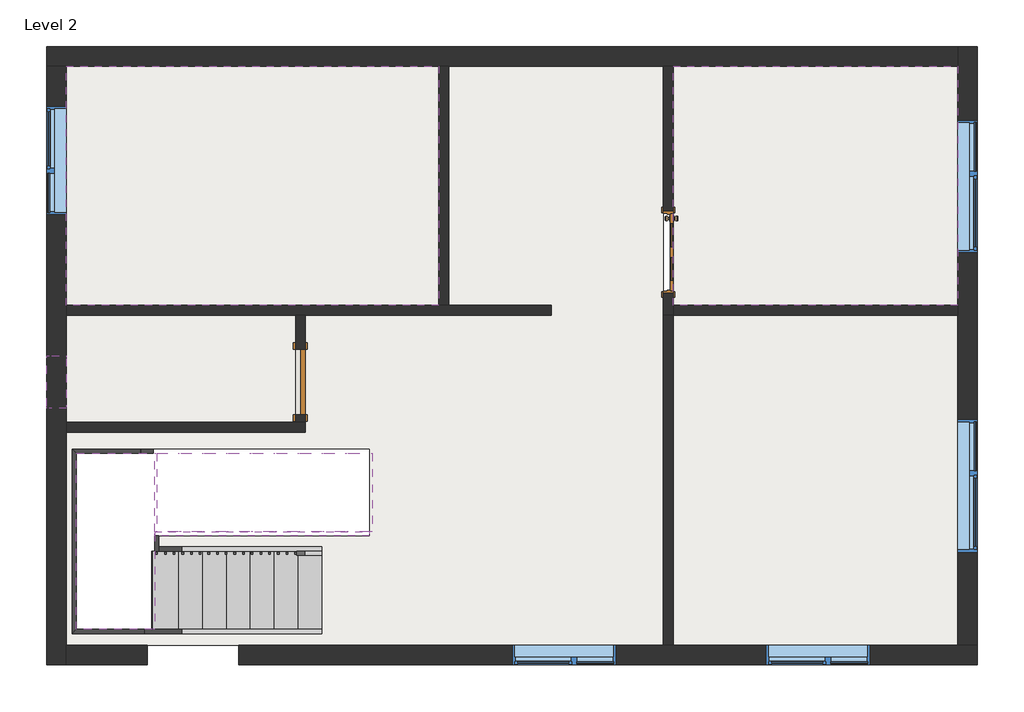
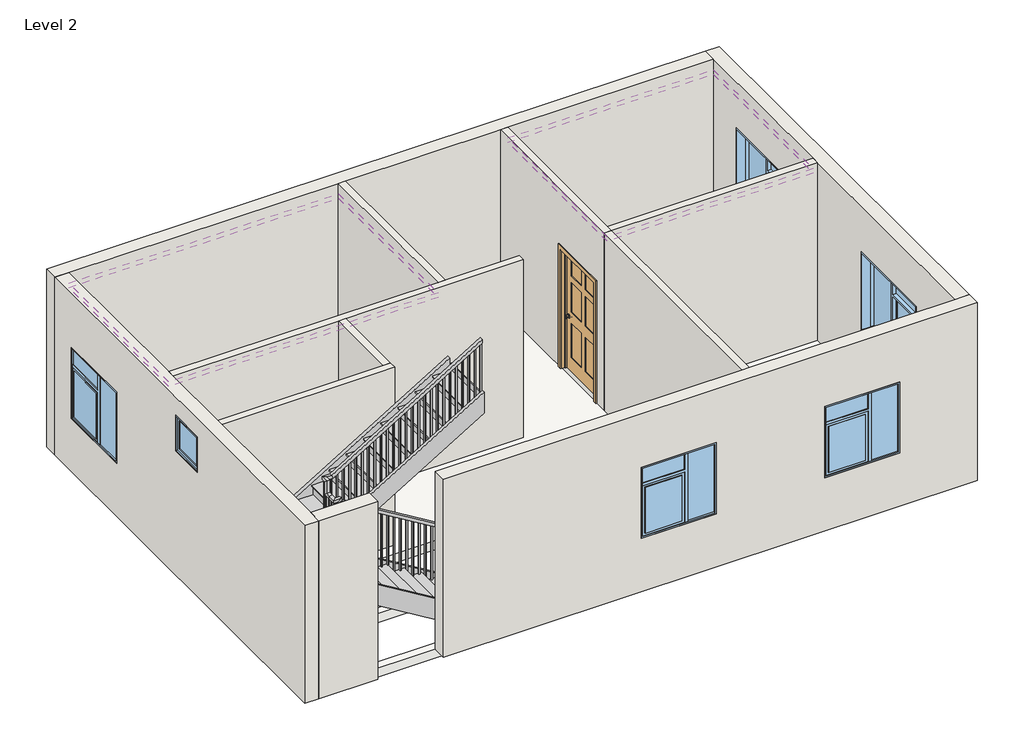
# One storey: 11 walls, 8 members, 6 windows, 4 coverings, 2 doors, 2 slabs, 2 stair flights, 1 railing.
"""IFC4 building model written with IfcOpenShell, lengths in millimetres."""

from ifc_helpers import new_model, si_unit, frame, origin, place, context, project, spatial, polyline, outline, extrude, faceted_brep, transform, mapped, element, save
from components import door_92bad2d9, door_d8f5dbb5, non_monolithic_landing_0199e9fe, stair_flight_13fda11b, stair_flight_c7e5c723, window_80340324, window_ae1cb28a, window_390faff0, window_casement_double_sidelight_windows_4_x_4_2_a48be683

model = new_model("IFC4")

# Units and contexts
model_context = context("Model", 3, world=origin())
ifc_project = project(units=[si_unit("LENGTHUNIT", "METRE", prefix="MILLI")], contexts=[model_context])

# Site, building, storey
site = spatial("IfcSite", under=ifc_project)
building = spatial("IfcBuilding", under=site)
storey = spatial("IfcBuildingStorey", under=building, Name="Level 2", Elevation=3352.8)

# Coverings
placement = place(None, origin())
element("IfcCovering", 1, ObjectType="METAL WHITE CEILING", at=placement, inside=storey, context=model_context, shape_type="SweptSolid", body=[
    extrude(outline(polyline([(-15611.0277023, 6236.3679075), (-11248.5777023, 6236.3679075), (-11248.5777023, 3436.0179075), (-15611.0277023, 3436.0179075), (-15611.0277023, 6236.3679075)])), frame((0.0, 0.0, 6223.0), z_axis=(0.0, 0.0, 1.0), x_axis=(1.0, 0.0, 0.0)), (0.0, 0.0, 1.0), 107.95),
])
element("IfcCovering", 2, ObjectType="METAL WHITE CEILING", at=placement, inside=storey, context=model_context, shape_type="SweptSolid", body=[
    extrude(outline(polyline([(-11248.5777023, 6236.3679075), (-11248.5777023, 3436.0179075), (-15611.0277023, 3436.0179075), (-15611.0277023, 6236.3679075), (-11248.5777023, 6236.3679075)]), holes=[polyline([(-11553.3777023, 5931.5679075), (-15306.2277023, 5931.5679075), (-15306.2277023, 3740.8179075), (-11553.3777023, 3740.8179075), (-11553.3777023, 5931.5679075)])]), frame((0.0, 0.0, 6146.8), z_axis=(0.0, 0.0, 1.0), x_axis=(1.0, 0.0, 0.0)), (0.0, 0.0, 1.0), 107.95),
    extrude(outline(polyline([(-14689.9397973, 5626.7679075), (-14689.9397973, 4045.6179075), (-15001.4277023, 4045.6179075), (-15001.4277023, 5626.7679075), (-14689.9397973, 5626.7679075)])), frame((0.0, 0.0, 6146.8), z_axis=(0.0, 0.0, 1.0), x_axis=(1.0, 0.0, 0.0)), (0.0, 0.0, 1.0), 107.95),
    extrude(outline(polyline([(-14080.3397973, 5626.7679075), (-14080.3397973, 4045.6179075), (-14391.8277023, 4045.6179075), (-14391.8277023, 5626.7679075), (-14080.3397973, 5626.7679075)])), frame((0.0, 0.0, 6146.8), z_axis=(0.0, 0.0, 1.0), x_axis=(1.0, 0.0, 0.0)), (0.0, 0.0, 1.0), 107.95),
    extrude(outline(polyline([(-13470.7397973, 5626.7679075), (-13470.7397973, 4045.6179075), (-13782.2277023, 4045.6179075), (-13782.2277023, 5626.7679075), (-13470.7397973, 5626.7679075)])), frame((0.0, 0.0, 6146.8), z_axis=(0.0, 0.0, 1.0), x_axis=(1.0, 0.0, 0.0)), (0.0, 0.0, 1.0), 107.95),
    extrude(outline(polyline([(-12861.1397973, 5626.7679075), (-12861.1397973, 4045.6179075), (-13172.6277023, 4045.6179075), (-13172.6277023, 5626.7679075), (-12861.1397973, 5626.7679075)])), frame((0.0, 0.0, 6146.8), z_axis=(0.0, 0.0, 1.0), x_axis=(1.0, 0.0, 0.0)), (0.0, 0.0, 1.0), 107.95),
    extrude(outline(polyline([(-12251.5397973, 5626.7679075), (-12251.5397973, 4045.6179075), (-12563.0277023, 4045.6179075), (-12563.0277023, 5626.7679075), (-12251.5397973, 5626.7679075)])), frame((0.0, 0.0, 6146.8), z_axis=(0.0, 0.0, 1.0), x_axis=(1.0, 0.0, 0.0)), (0.0, 0.0, 1.0), 107.95),
    extrude(outline(polyline([(-11641.9397973, 5626.7679075), (-11641.9397973, 4045.6179075), (-11953.4277023, 4045.6179075), (-11953.4277023, 5626.7679075), (-11641.9397973, 5626.7679075)])), frame((0.0, 0.0, 6146.8), z_axis=(0.0, 0.0, 1.0), x_axis=(1.0, 0.0, 0.0)), (0.0, 0.0, 1.0), 107.95),
])
element("IfcCovering", 3, ObjectType="METAL WHITE CEILING", at=placement, inside=storey, context=model_context, shape_type="SweptSolid", body=[
    extrude(outline(polyline([(-8505.3777023, 3436.0179075), (-8505.3777023, 6236.3679075), (-5171.6277023, 6236.3679075), (-5171.6277023, 3436.0179075), (-8505.3777023, 3436.0179075)])), frame((0.0, 0.0, 6223.0), z_axis=(0.0, 0.0, 1.0), x_axis=(1.0, 0.0, 0.0)), (0.0, 0.0, 1.0), 107.95),
])
element("IfcCovering", 4, ObjectType="METAL WHITE CEILING", at=placement, inside=storey, context=model_context, shape_type="SweptSolid", body=[
    extrude(outline(polyline([(-5171.6277023, 6236.3679075), (-5171.6277023, 3436.0179075), (-8505.3777023, 3436.0179075), (-8505.3777023, 6236.3679075), (-5171.6277023, 6236.3679075)]), holes=[polyline([(-5476.4277023, 5931.5679075), (-8200.5777023, 5931.5679075), (-8200.5777023, 3740.8179075), (-5476.4277023, 3740.8179075), (-5476.4277023, 5931.5679075)])]), frame((0.0, 0.0, 6146.8), z_axis=(0.0, 0.0, 1.0), x_axis=(1.0, 0.0, 0.0)), (0.0, 0.0, 1.0), 107.95),
    extrude(outline(polyline([(-7575.2115209, 5626.7679075), (-7575.2115209, 4045.6179075), (-7880.0115209, 4045.6179075), (-7880.0115209, 5626.7679075), (-7575.2115209, 5626.7679075)])), frame((0.0, 0.0, 6146.8), z_axis=(0.0, 0.0, 1.0), x_axis=(1.0, 0.0, 0.0)), (0.0, 0.0, 1.0), 107.95),
    extrude(outline(polyline([(-6965.6115209, 5626.7679075), (-6965.6115209, 4045.6179075), (-7270.4115209, 4045.6179075), (-7270.4115209, 5626.7679075), (-6965.6115209, 5626.7679075)])), frame((0.0, 0.0, 6146.8), z_axis=(0.0, 0.0, 1.0), x_axis=(1.0, 0.0, 0.0)), (0.0, 0.0, 1.0), 107.95),
    extrude(outline(polyline([(-6356.0115209, 5626.7679075), (-6356.0115209, 4045.6179075), (-6660.8115209, 4045.6179075), (-6660.8115209, 5626.7679075), (-6356.0115209, 5626.7679075)])), frame((0.0, 0.0, 6146.8), z_axis=(0.0, 0.0, 1.0), x_axis=(1.0, 0.0, 0.0)), (0.0, 0.0, 1.0), 107.95),
    extrude(outline(polyline([(-5746.4115209, 5626.7679075), (-5746.4115209, 4045.6179075), (-6051.2115209, 4045.6179075), (-6051.2115209, 5626.7679075), (-5746.4115209, 5626.7679075)])), frame((0.0, 0.0, 6146.8), z_axis=(0.0, 0.0, 1.0), x_axis=(1.0, 0.0, 0.0)), (0.0, 0.0, 1.0), 107.95),
])

# Doors
door_shape = door_92bad2d9(model_context)
element("IfcDoor", 5, ObjectType="Door-Interior-Single-6_Panel-Wood : 36\" x 80\"", at=placement, inside=storey, context=model_context, shape_type="MappedRepresentation", body=[
    mapped(door_shape, transform((-8559.3527023, 4058.3179075, 3352.8), x_axis=(0.0, -1.0, 0.0), y_axis=(1.0, 0.0, 0.0), z_axis=(0.0, 0.0, 1.0))),
])
door_2_shape = door_d8f5dbb5(model_context)
element("IfcDoor", 6, ObjectType="Single-Flush : 30\" x 80\"", at=placement, inside=storey, context=model_context, shape_type="MappedRepresentation", body=[
    mapped(door_2_shape, transform((-12867.8277023, 2538.826922, 3386.2495969), x_axis=(0.0, -1.0, 0.0), y_axis=(1.0, 0.0, 0.0), z_axis=(0.0, 0.0, 1.0))),
])

# Members
element("IfcMember", 7, ObjectType="Stringer - 2\" Width", at=placement, inside=storey, context=model_context, shape_type="SweptSolid", body=[
    extrude(outline(polyline([(3352.8, -12620.1777023), (3564.914512, -12620.1777023), (4783.6666667, -14631.1187576), (4478.8666667, -14716.2732141), (3352.8, -12858.2632141), (3352.8, -12620.1777023)])), frame((0.0, -405.7320925, 0.0), z_axis=(0.0, 1.0, 0.0), x_axis=(0.0, 0.0, 1.0)), (0.0, 0.0, 1.0), 50.8),
])
element("IfcMember", 8, ObjectType="Stringer - 2\" Width", at=placement, inside=storey, context=model_context, shape_type="SweptSolid", body=[
    extrude(outline(polyline([(3352.8, -12620.1777023), (3564.914512, -12620.1777023), (4719.4599665, -14525.1777023), (4363.051205, -14525.1777023), (3352.8, -12858.2632141), (3352.8, -12620.1777023)])), frame((0.0, 559.4679075, 0.0), z_axis=(0.0, 1.0, 0.0), x_axis=(0.0, 0.0, 1.0)), (0.0, 0.0, 1.0), 50.8),
])
element("IfcMember", 9, ObjectType="Stringer - 2\" Width", at=placement, inside=storey, context=model_context, shape_type="SweptSolid", body=[
    extrude(outline(polyline([(4783.6666667, -14800.2366471), (4478.8666667, -14715.0821905), (6087.1724171, -12061.3777023), (6443.5811786, -12061.3777023), (4783.6666667, -14800.2366471)])), frame((0.0, 1702.4679075, 0.0), z_axis=(0.0, 1.0, 0.0), x_axis=(0.0, 0.0, 1.0)), (0.0, 0.0, 1.0), 50.8),
])
element("IfcMember", 10, ObjectType="Stringer - 2\" Width", at=placement, inside=storey, context=model_context, shape_type="SweptSolid", body=[
    extrude(outline(polyline([(4919.5811786, -14575.9777023), (4563.1724171, -14575.9777023), (6087.1724171, -12061.3777023), (6443.5811786, -12061.3777023), (4919.5811786, -14575.9777023)])), frame((0.0, 737.2679075, 0.0), z_axis=(0.0, 1.0, 0.0), x_axis=(0.0, 0.0, 1.0)), (0.0, 0.0, 1.0), 50.8),
])
element("IfcMember", 11, ObjectType="Stringer - 2\" Width", at=placement, inside=storey, context=model_context, shape_type="Brep", body=[
    faceted_brep([(-14800.2366471, 1702.4679075, 4783.6666667), (-14800.2366471, 1753.2679075, 4783.6666667), (-15541.1777023, 1753.2679075, 4783.6666667), (-15490.3777023, 1702.4679075, 4783.6666667), (-14715.0821905, 1702.4679075, 4478.8666667), (-15490.3777023, 1702.4679075, 4478.8666667), (-14715.0821905, 1753.2679075, 4478.8666667), (-15541.1777023, 1753.2679075, 4478.8666667)], [[[0, 1, 2, 3]], [[4, 0, 3, 5]], [[6, 4, 5, 7]], [[1, 6, 7, 2]], [[1, 0, 4, 6]], [[2, 7, 5, 3]]]),
])
element("IfcMember", 12, ObjectType="Stringer - 2\" Width", at=placement, inside=storey, context=model_context, shape_type="SweptSolid", body=[
    extrude(outline(polyline([(-15541.1777023, 1753.2679075), (-15490.3777023, 1702.4679075), (-15490.3777023, -354.9320925), (-15541.1777023, -405.7320925), (-15541.1777023, 1753.2679075)])), frame((0.0, 0.0, 4478.8666667), z_axis=(0.0, 0.0, 1.0), x_axis=(1.0, 0.0, 0.0)), (0.0, 0.0, 1.0), 304.8),
])
element("IfcMember", 13, ObjectType="Stringer - 2\" Width", at=placement, inside=storey, context=model_context, shape_type="Brep", body=[
    faceted_brep([(-15490.3777023, -354.9320925, 4783.6666667), (-15541.1777023, -405.7320925, 4783.6666667), (-14631.1187576, -405.7320925, 4783.6666667), (-14631.1187576, -354.9320925, 4783.6666667), (-15490.3777023, -354.9320925, 4478.8666667), (-14716.2732141, -354.9320925, 4478.8666667), (-15541.1777023, -405.7320925, 4478.8666667), (-14716.2732141, -405.7320925, 4478.8666667)], [[[0, 1, 2, 3]], [[4, 0, 3, 5]], [[6, 4, 5, 7]], [[1, 6, 7, 2]], [[1, 0, 4, 6]], [[2, 7, 5, 3]]]),
])
element("IfcMember", 14, ObjectType="Stringer - 2\" Width", at=placement, inside=storey, context=model_context, shape_type="SweptSolid", body=[
    extrude(outline(polyline([(-14525.1777023, 559.4679075), (-14575.9777023, 559.4679075), (-14575.9777023, 737.2679075), (-14525.1777023, 737.2679075), (-14525.1777023, 559.4679075)])), frame((0.0, 0.0, 4478.8666667), z_axis=(0.0, 0.0, 1.0), x_axis=(1.0, 0.0, 0.0)), (0.0, 0.0, 1.0), 304.8),
])

# Railing
element("IfcRailing", 15, ObjectType="Handrail - Rectangular", at=placement, inside=storey, context=model_context, shape_type="SolidModel", body=[
    faceted_brep([(-12620.1777023, 508.6679075, 4436.5333333), (-12620.1777023, 508.6679075, 4377.1318731), (-12620.1777023, 559.4679075, 4377.1318731), (-12620.1777023, 559.4679075, 4436.5333333), (-14499.7777023, 508.6679075, 5575.6848485), (-14550.5777023, 508.6679075, 5547.071267), (-14550.5777023, 559.4679075, 5547.071267), (-14499.7777023, 559.4679075, 5575.6848485), (-14499.7777023, 508.6679075, 5621.8666667), (-14550.5777023, 508.6679075, 5571.0666667), (-14550.5777023, 559.4679075, 5571.0666667), (-14499.7777023, 559.4679075, 5621.8666667), (-14626.7777023, 508.6679075, 5621.8666667), (-14626.7777023, 508.6679075, 5571.0666667), (-14575.9777023, 559.4679075, 5571.0666667), (-14575.9777023, 559.4679075, 5621.8666667), (-14626.7777023, 635.6679075, 5621.8666667), (-14626.7777023, 635.6679075, 5571.0666667), (-14575.9777023, 635.6679075, 5571.0666667), (-14575.9777023, 635.6679075, 5621.8666667), (-14626.7777023, 711.8679075, 5621.8666667), (-14626.7777023, 762.6679075, 5571.0666667), (-14575.9777023, 762.6679075, 5571.0666667), (-14575.9777023, 711.8679075, 5621.8666667), (-14626.7777023, 711.8679075, 5837.3818182), (-14626.7777023, 762.6679075, 5786.5818182), (-14575.9777023, 762.6679075, 5786.5818182), (-14575.9777023, 711.8679075, 5837.3818182), (-14626.7777023, 838.8679075, 5837.3818182), (-14626.7777023, 838.8679075, 5786.5818182), (-14575.9777023, 788.0679075, 5786.5818182), (-14575.9777023, 788.0679075, 5837.3818182), (-14499.7777023, 838.8679075, 5837.3818182), (-14485.5852929, 838.8679075, 5786.5818182), (-14485.5852929, 788.0679075, 5786.5818182), (-14499.7777023, 788.0679075, 5837.3818182), (-12061.3777023, 838.8679075, 7315.2), (-12061.3777023, 788.0679075, 7315.2), (-12061.3777023, 788.0679075, 7255.7985397), (-12061.3777023, 838.8679075, 7255.7985397)], [[[0, 1, 2, 3]], [[1, 0, 4, 5]], [[2, 1, 5, 6]], [[3, 2, 6, 7]], [[0, 3, 7, 4]], [[5, 4, 8, 9]], [[6, 5, 9, 10]], [[7, 6, 10, 11]], [[4, 7, 11, 8]], [[9, 8, 12, 13]], [[10, 9, 13, 14]], [[11, 10, 14, 15]], [[8, 11, 15, 12]], [[13, 12, 16, 17]], [[14, 13, 17, 18]], [[15, 14, 18, 19]], [[12, 15, 19, 16]], [[17, 16, 20, 21]], [[18, 17, 21, 22]], [[19, 18, 22, 23]], [[16, 19, 23, 20]], [[21, 20, 24, 25]], [[22, 21, 25, 26]], [[23, 22, 26, 27]], [[20, 23, 27, 24]], [[25, 24, 28, 29]], [[26, 25, 29, 30]], [[27, 26, 30, 31]], [[24, 27, 31, 28]], [[29, 28, 32, 33]], [[30, 29, 33, 34]], [[31, 30, 34, 35]], [[28, 31, 35, 32]], [[36, 37, 38, 39]], [[33, 32, 36, 39]], [[34, 33, 39, 38]], [[35, 34, 38, 37]], [[32, 35, 37, 36]]]),
    extrude(outline(polyline([(7199.9955094, -12153.4527023), (7188.4500549, -12172.5027023), (6231.4666667, -12172.5027023), (6231.4666667, -12153.4527023), (7199.9955094, -12153.4527023)])), frame((0.0, 803.9429075, 0.0), z_axis=(0.0, 1.0, 0.0), x_axis=(0.0, 0.0, 1.0)), (0.0, 0.0, 1.0), 19.05),
    extrude(outline(polyline([(7138.4197519, -12255.0527023), (7126.8742973, -12274.1027023), (6231.4666667, -12274.1027023), (6231.4666667, -12255.0527023), (7138.4197519, -12255.0527023)])), frame((0.0, 803.9429075, 0.0), z_axis=(0.0, 1.0, 0.0), x_axis=(0.0, 0.0, 1.0)), (0.0, 0.0, 1.0), 19.05),
    extrude(outline(polyline([(7076.8439943, -12356.6527023), (7065.2985397, -12375.7027023), (6062.1333333, -12375.7027023), (6062.1333333, -12356.6527023), (7076.8439943, -12356.6527023)])), frame((0.0, 803.9429075, 0.0), z_axis=(0.0, 1.0, 0.0), x_axis=(0.0, 0.0, 1.0)), (0.0, 0.0, 1.0), 19.05),
    extrude(outline(polyline([(7015.2682367, -12458.2527023), (7003.7227822, -12477.3027023), (6062.1333333, -12477.3027023), (6062.1333333, -12458.2527023), (7015.2682367, -12458.2527023)])), frame((0.0, 803.9429075, 0.0), z_axis=(0.0, 1.0, 0.0), x_axis=(0.0, 0.0, 1.0)), (0.0, 0.0, 1.0), 19.05),
    extrude(outline(polyline([(6953.6924791, -12559.8527023), (6942.1470246, -12578.9027023), (6062.1333333, -12578.9027023), (6062.1333333, -12559.8527023), (6953.6924791, -12559.8527023)])), frame((0.0, 803.9429075, 0.0), z_axis=(0.0, 1.0, 0.0), x_axis=(0.0, 0.0, 1.0)), (0.0, 0.0, 1.0), 19.05),
    extrude(outline(polyline([(6892.1167216, -12661.4527023), (6880.571267, -12680.5027023), (5892.8, -12680.5027023), (5892.8, -12661.4527023), (6892.1167216, -12661.4527023)])), frame((0.0, 803.9429075, 0.0), z_axis=(0.0, 1.0, 0.0), x_axis=(0.0, 0.0, 1.0)), (0.0, 0.0, 1.0), 19.05),
    extrude(outline(polyline([(6830.540964, -12763.0527023), (6818.9955094, -12782.1027023), (5892.8, -12782.1027023), (5892.8, -12763.0527023), (6830.540964, -12763.0527023)])), frame((0.0, 803.9429075, 0.0), z_axis=(0.0, 1.0, 0.0), x_axis=(0.0, 0.0, 1.0)), (0.0, 0.0, 1.0), 19.05),
    extrude(outline(polyline([(6768.9652064, -12864.6527023), (6757.4197519, -12883.7027023), (5892.8, -12883.7027023), (5892.8, -12864.6527023), (6768.9652064, -12864.6527023)])), frame((0.0, 803.9429075, 0.0), z_axis=(0.0, 1.0, 0.0), x_axis=(0.0, 0.0, 1.0)), (0.0, 0.0, 1.0), 19.05),
    extrude(outline(polyline([(6707.3894488, -12966.2527023), (6695.8439943, -12985.3027023), (5723.4666667, -12985.3027023), (5723.4666667, -12966.2527023), (6707.3894488, -12966.2527023)])), frame((0.0, 803.9429075, 0.0), z_axis=(0.0, 1.0, 0.0), x_axis=(0.0, 0.0, 1.0)), (0.0, 0.0, 1.0), 19.05),
    extrude(outline(polyline([(6645.8136913, -13067.8527023), (6634.2682367, -13086.9027023), (5723.4666667, -13086.9027023), (5723.4666667, -13067.8527023), (6645.8136913, -13067.8527023)])), frame((0.0, 803.9429075, 0.0), z_axis=(0.0, 1.0, 0.0), x_axis=(0.0, 0.0, 1.0)), (0.0, 0.0, 1.0), 19.05),
    extrude(outline(polyline([(6584.2379337, -13169.4527023), (6572.6924791, -13188.5027023), (5723.4666667, -13188.5027023), (5723.4666667, -13169.4527023), (6584.2379337, -13169.4527023)])), frame((0.0, 803.9429075, 0.0), z_axis=(0.0, 1.0, 0.0), x_axis=(0.0, 0.0, 1.0)), (0.0, 0.0, 1.0), 19.05),
    extrude(outline(polyline([(6522.6621761, -13271.0527023), (6511.1167216, -13290.1027023), (5554.1333333, -13290.1027023), (5554.1333333, -13271.0527023), (6522.6621761, -13271.0527023)])), frame((0.0, 803.9429075, 0.0), z_axis=(0.0, 1.0, 0.0), x_axis=(0.0, 0.0, 1.0)), (0.0, 0.0, 1.0), 19.05),
    extrude(outline(polyline([(6461.0864185, -13372.6527023), (6449.540964, -13391.7027023), (5554.1333333, -13391.7027023), (5554.1333333, -13372.6527023), (6461.0864185, -13372.6527023)])), frame((0.0, 803.9429075, 0.0), z_axis=(0.0, 1.0, 0.0), x_axis=(0.0, 0.0, 1.0)), (0.0, 0.0, 1.0), 19.05),
    extrude(outline(polyline([(6399.510661, -13474.2527023), (6387.9652064, -13493.3027023), (5384.8, -13493.3027023), (5384.8, -13474.2527023), (6399.510661, -13474.2527023)])), frame((0.0, 803.9429075, 0.0), z_axis=(0.0, 1.0, 0.0), x_axis=(0.0, 0.0, 1.0)), (0.0, 0.0, 1.0), 19.05),
    extrude(outline(polyline([(6337.9349034, -13575.8527023), (6326.3894488, -13594.9027023), (5384.8, -13594.9027023), (5384.8, -13575.8527023), (6337.9349034, -13575.8527023)])), frame((0.0, 803.9429075, 0.0), z_axis=(0.0, 1.0, 0.0), x_axis=(0.0, 0.0, 1.0)), (0.0, 0.0, 1.0), 19.05),
    extrude(outline(polyline([(6276.3591458, -13677.4527023), (6264.8136913, -13696.5027023), (5384.8, -13696.5027023), (5384.8, -13677.4527023), (6276.3591458, -13677.4527023)])), frame((0.0, 803.9429075, 0.0), z_axis=(0.0, 1.0, 0.0), x_axis=(0.0, 0.0, 1.0)), (0.0, 0.0, 1.0), 19.05),
    extrude(outline(polyline([(6214.7833882, -13779.0527023), (6203.2379337, -13798.1027023), (5215.4666667, -13798.1027023), (5215.4666667, -13779.0527023), (6214.7833882, -13779.0527023)])), frame((0.0, 803.9429075, 0.0), z_axis=(0.0, 1.0, 0.0), x_axis=(0.0, 0.0, 1.0)), (0.0, 0.0, 1.0), 19.05),
    extrude(outline(polyline([(6153.2076307, -13880.6527023), (6141.6621761, -13899.7027023), (5215.4666667, -13899.7027023), (5215.4666667, -13880.6527023), (6153.2076307, -13880.6527023)])), frame((0.0, 803.9429075, 0.0), z_axis=(0.0, 1.0, 0.0), x_axis=(0.0, 0.0, 1.0)), (0.0, 0.0, 1.0), 19.05),
    extrude(outline(polyline([(6091.6318731, -13982.2527023), (6080.0864185, -14001.3027023), (5215.4666667, -14001.3027023), (5215.4666667, -13982.2527023), (6091.6318731, -13982.2527023)])), frame((0.0, 803.9429075, 0.0), z_axis=(0.0, 1.0, 0.0), x_axis=(0.0, 0.0, 1.0)), (0.0, 0.0, 1.0), 19.05),
    extrude(outline(polyline([(6030.0561155, -14083.8527023), (6018.510661, -14102.9027023), (5046.1333333, -14102.9027023), (5046.1333333, -14083.8527023), (6030.0561155, -14083.8527023)])), frame((0.0, 803.9429075, 0.0), z_axis=(0.0, 1.0, 0.0), x_axis=(0.0, 0.0, 1.0)), (0.0, 0.0, 1.0), 19.05),
    extrude(outline(polyline([(5968.4803579, -14185.4527023), (5956.9349034, -14204.5027023), (5046.1333333, -14204.5027023), (5046.1333333, -14185.4527023), (5968.4803579, -14185.4527023)])), frame((0.0, 803.9429075, 0.0), z_axis=(0.0, 1.0, 0.0), x_axis=(0.0, 0.0, 1.0)), (0.0, 0.0, 1.0), 19.05),
    extrude(outline(polyline([(5906.9046004, -14287.0527023), (5895.3591458, -14306.1027023), (5046.1333333, -14306.1027023), (5046.1333333, -14287.0527023), (5906.9046004, -14287.0527023)])), frame((0.0, 803.9429075, 0.0), z_axis=(0.0, 1.0, 0.0), x_axis=(0.0, 0.0, 1.0)), (0.0, 0.0, 1.0), 19.05),
    extrude(outline(polyline([(5845.3288428, -14388.6527023), (5833.7833882, -14407.7027023), (4876.8, -14407.7027023), (4876.8, -14388.6527023), (5845.3288428, -14388.6527023)])), frame((0.0, 803.9429075, 0.0), z_axis=(0.0, 1.0, 0.0), x_axis=(0.0, 0.0, 1.0)), (0.0, 0.0, 1.0), 19.05),
    extrude(outline(polyline([(5783.7530852, -14490.2527023), (5772.2076307, -14509.3027023), (4876.8, -14509.3027023), (4876.8, -14490.2527023), (5783.7530852, -14490.2527023)])), frame((0.0, 803.9429075, 0.0), z_axis=(0.0, 1.0, 0.0), x_axis=(0.0, 0.0, 1.0)), (0.0, 0.0, 1.0), 19.05),
    extrude(outline(polyline([(-14591.8527023, 727.7429075), (-14610.9027023, 727.7429075), (-14610.9027023, 746.7929075), (-14591.8527023, 746.7929075), (-14591.8527023, 727.7429075)])), frame((0.0, 0.0, 4707.4666667), z_axis=(0.0, 0.0, 1.0), x_axis=(1.0, 0.0, 0.0)), (0.0, 0.0, 1.0), 1079.1151515),
    extrude(outline(polyline([(-14591.8527023, 626.1429075), (-14610.9027023, 626.1429075), (-14610.9027023, 645.1929075), (-14591.8527023, 645.1929075), (-14591.8527023, 626.1429075)])), frame((0.0, 0.0, 4707.4666667), z_axis=(0.0, 0.0, 1.0), x_axis=(1.0, 0.0, 0.0)), (0.0, 0.0, 1.0), 863.6),
    extrude(outline(polyline([(-14541.0527023, 543.5929075), (-14541.0527023, 524.5429075), (-14560.1027023, 524.5429075), (-14560.1027023, 543.5929075), (-14541.0527023, 543.5929075)])), frame((0.0, 0.0, 4538.1333333), z_axis=(0.0, 0.0, 1.0), x_axis=(1.0, 0.0, 0.0)), (0.0, 0.0, 1.0), 1032.9333333),
    extrude(outline(polyline([(5479.7227822, -14439.4527023), (5491.2682367, -14458.5027023), (4538.1333333, -14458.5027023), (4538.1333333, -14439.4527023), (5479.7227822, -14439.4527023)])), frame((0.0, 524.5429075, 0.0), z_axis=(0.0, 1.0, 0.0), x_axis=(0.0, 0.0, 1.0)), (0.0, 0.0, 1.0), 19.05),
    extrude(outline(polyline([(5418.1470246, -14337.8527023), (5429.6924791, -14356.9027023), (4538.1333333, -14356.9027023), (4538.1333333, -14337.8527023), (5418.1470246, -14337.8527023)])), frame((0.0, 524.5429075, 0.0), z_axis=(0.0, 1.0, 0.0), x_axis=(0.0, 0.0, 1.0)), (0.0, 0.0, 1.0), 19.05),
    extrude(outline(polyline([(5356.571267, -14236.2527023), (5368.1167216, -14255.3027023), (4368.8, -14255.3027023), (4368.8, -14236.2527023), (5356.571267, -14236.2527023)])), frame((0.0, 524.5429075, 0.0), z_axis=(0.0, 1.0, 0.0), x_axis=(0.0, 0.0, 1.0)), (0.0, 0.0, 1.0), 19.05),
    extrude(outline(polyline([(5294.9955094, -14134.6527023), (5306.540964, -14153.7027023), (4368.8, -14153.7027023), (4368.8, -14134.6527023), (5294.9955094, -14134.6527023)])), frame((0.0, 524.5429075, 0.0), z_axis=(0.0, 1.0, 0.0), x_axis=(0.0, 0.0, 1.0)), (0.0, 0.0, 1.0), 19.05),
    extrude(outline(polyline([(5233.4197519, -14033.0527023), (5244.9652064, -14052.1027023), (4368.8, -14052.1027023), (4368.8, -14033.0527023), (5233.4197519, -14033.0527023)])), frame((0.0, 524.5429075, 0.0), z_axis=(0.0, 1.0, 0.0), x_axis=(0.0, 0.0, 1.0)), (0.0, 0.0, 1.0), 19.05),
    extrude(outline(polyline([(5171.8439943, -13931.4527023), (5183.3894488, -13950.5027023), (4199.4666667, -13950.5027023), (4199.4666667, -13931.4527023), (5171.8439943, -13931.4527023)])), frame((0.0, 524.5429075, 0.0), z_axis=(0.0, 1.0, 0.0), x_axis=(0.0, 0.0, 1.0)), (0.0, 0.0, 1.0), 19.05),
    extrude(outline(polyline([(5110.2682367, -13829.8527023), (5121.8136913, -13848.9027023), (4199.4666667, -13848.9027023), (4199.4666667, -13829.8527023), (5110.2682367, -13829.8527023)])), frame((0.0, 524.5429075, 0.0), z_axis=(0.0, 1.0, 0.0), x_axis=(0.0, 0.0, 1.0)), (0.0, 0.0, 1.0), 19.05),
    extrude(outline(polyline([(5048.6924791, -13728.2527023), (5060.2379337, -13747.3027023), (4199.4666667, -13747.3027023), (4199.4666667, -13728.2527023), (5048.6924791, -13728.2527023)])), frame((0.0, 524.5429075, 0.0), z_axis=(0.0, 1.0, 0.0), x_axis=(0.0, 0.0, 1.0)), (0.0, 0.0, 1.0), 19.05),
    extrude(outline(polyline([(4987.1167216, -13626.6527023), (4998.6621761, -13645.7027023), (4030.1333333, -13645.7027023), (4030.1333333, -13626.6527023), (4987.1167216, -13626.6527023)])), frame((0.0, 524.5429075, 0.0), z_axis=(0.0, 1.0, 0.0), x_axis=(0.0, 0.0, 1.0)), (0.0, 0.0, 1.0), 19.05),
    extrude(outline(polyline([(4925.540964, -13525.0527023), (4937.0864185, -13544.1027023), (4030.1333333, -13544.1027023), (4030.1333333, -13525.0527023), (4925.540964, -13525.0527023)])), frame((0.0, 524.5429075, 0.0), z_axis=(0.0, 1.0, 0.0), x_axis=(0.0, 0.0, 1.0)), (0.0, 0.0, 1.0), 19.05),
    extrude(outline(polyline([(4863.9652064, -13423.4527023), (4875.510661, -13442.5027023), (3860.8, -13442.5027023), (3860.8, -13423.4527023), (4863.9652064, -13423.4527023)])), frame((0.0, 524.5429075, 0.0), z_axis=(0.0, 1.0, 0.0), x_axis=(0.0, 0.0, 1.0)), (0.0, 0.0, 1.0), 19.05),
    extrude(outline(polyline([(4802.3894488, -13321.8527023), (4813.9349034, -13340.9027023), (3860.8, -13340.9027023), (3860.8, -13321.8527023), (4802.3894488, -13321.8527023)])), frame((0.0, 524.5429075, 0.0), z_axis=(0.0, 1.0, 0.0), x_axis=(0.0, 0.0, 1.0)), (0.0, 0.0, 1.0), 19.05),
    extrude(outline(polyline([(4740.8136913, -13220.2527023), (4752.3591458, -13239.3027023), (3860.8, -13239.3027023), (3860.8, -13220.2527023), (4740.8136913, -13220.2527023)])), frame((0.0, 524.5429075, 0.0), z_axis=(0.0, 1.0, 0.0), x_axis=(0.0, 0.0, 1.0)), (0.0, 0.0, 1.0), 19.05),
    extrude(outline(polyline([(4679.2379337, -13118.6527023), (4690.7833882, -13137.7027023), (3691.4666667, -13137.7027023), (3691.4666667, -13118.6527023), (4679.2379337, -13118.6527023)])), frame((0.0, 524.5429075, 0.0), z_axis=(0.0, 1.0, 0.0), x_axis=(0.0, 0.0, 1.0)), (0.0, 0.0, 1.0), 19.05),
    extrude(outline(polyline([(4617.6621761, -13017.0527023), (4629.2076307, -13036.1027023), (3691.4666667, -13036.1027023), (3691.4666667, -13017.0527023), (4617.6621761, -13017.0527023)])), frame((0.0, 524.5429075, 0.0), z_axis=(0.0, 1.0, 0.0), x_axis=(0.0, 0.0, 1.0)), (0.0, 0.0, 1.0), 19.05),
    extrude(outline(polyline([(4556.0864185, -12915.4527023), (4567.6318731, -12934.5027023), (3691.4666667, -12934.5027023), (3691.4666667, -12915.4527023), (4556.0864185, -12915.4527023)])), frame((0.0, 524.5429075, 0.0), z_axis=(0.0, 1.0, 0.0), x_axis=(0.0, 0.0, 1.0)), (0.0, 0.0, 1.0), 19.05),
    extrude(outline(polyline([(4494.510661, -12813.8527023), (4506.0561155, -12832.9027023), (3522.1333333, -12832.9027023), (3522.1333333, -12813.8527023), (4494.510661, -12813.8527023)])), frame((0.0, 524.5429075, 0.0), z_axis=(0.0, 1.0, 0.0), x_axis=(0.0, 0.0, 1.0)), (0.0, 0.0, 1.0), 19.05),
    extrude(outline(polyline([(4432.9349034, -12712.2527023), (4444.4803579, -12731.3027023), (3522.1333333, -12731.3027023), (3522.1333333, -12712.2527023), (4432.9349034, -12712.2527023)])), frame((0.0, 524.5429075, 0.0), z_axis=(0.0, 1.0, 0.0), x_axis=(0.0, 0.0, 1.0)), (0.0, 0.0, 1.0), 19.05),
    extrude(outline(polyline([(-14591.8527023, 803.9429075), (-14610.9027023, 803.9429075), (-14610.9027023, 822.9929075), (-14591.8527023, 822.9929075), (-14591.8527023, 803.9429075)])), frame((0.0, 0.0, 4707.4666667), z_axis=(0.0, 0.0, 1.0), x_axis=(1.0, 0.0, 0.0)), (0.0, 0.0, 1.0), 1079.1151515),
    extrude(outline(polyline([(-14591.8527023, 543.5929075), (-14591.8527023, 524.5429075), (-14610.9027023, 524.5429075), (-14610.9027023, 543.5929075), (-14591.8527023, 543.5929075)])), frame((0.0, 0.0, 4707.4666667), z_axis=(0.0, 0.0, 1.0), x_axis=(1.0, 0.0, 0.0)), (0.0, 0.0, 1.0), 863.6),
    extrude(outline(polyline([(7255.7985397, -12061.3777023), (7244.2530852, -12080.4277023), (6231.4666667, -12080.4277023), (6231.4666667, -12061.3777023), (7255.7985397, -12061.3777023)])), frame((0.0, 803.9429075, 0.0), z_axis=(0.0, 1.0, 0.0), x_axis=(0.0, 0.0, 1.0)), (0.0, 0.0, 1.0), 19.05),
    extrude(outline(polyline([(4377.1318731, -12620.1777023), (4388.6773276, -12639.2277023), (3522.1333333, -12639.2277023), (3522.1333333, -12620.1777023), (4377.1318731, -12620.1777023)])), frame((0.0, 524.5429075, 0.0), z_axis=(0.0, 1.0, 0.0), x_axis=(0.0, 0.0, 1.0)), (0.0, 0.0, 1.0), 19.05),
])

# Slabs
element("IfcSlab", 16, ObjectType="FLOORING 6\"", at=placement, inside=storey, context=model_context, shape_type="SweptSolid", body=[
    extrude(outline(polyline([(-11248.5777023, 6236.3679075), (-11248.5777023, 3436.0179075), (-15611.0277023, 3436.0179075), (-15611.0277023, 6236.3679075), (-11248.5777023, 6236.3679075)])), frame((0.0, 0.0, 3200.4), z_axis=(0.0, 0.0, 1.0), x_axis=(1.0, 0.0, 0.0)), (0.0, 0.0, 1.0), 152.4),
    extrude(outline(polyline([(-5171.6277023, 6236.3679075), (-5171.6277023, 3436.0179075), (-8505.3777023, 3436.0179075), (-8505.3777023, 6236.3679075), (-5171.6277023, 6236.3679075)])), frame((0.0, 0.0, 3200.4), z_axis=(0.0, 0.0, 1.0), x_axis=(1.0, 0.0, 0.0)), (0.0, 0.0, 1.0), 152.4),
    extrude(outline(polyline([(-5171.6277023, 3321.7179075), (-5171.6277023, -545.4320925), (-8505.3777023, -545.4320925), (-8505.3777023, 3321.7179075), (-5171.6277023, 3321.7179075)])), frame((0.0, 0.0, 3200.4), z_axis=(0.0, 0.0, 1.0), x_axis=(1.0, 0.0, 0.0)), (0.0, 0.0, 1.0), 152.4),
    extrude(outline(polyline([(-12924.9777023, 3321.7179075), (-12924.9777023, 2064.4179075), (-15611.0277023, 2064.4179075), (-15611.0277023, 3321.7179075), (-12924.9777023, 3321.7179075)])), frame((0.0, 0.0, 3200.4), z_axis=(0.0, 0.0, 1.0), x_axis=(1.0, 0.0, 0.0)), (0.0, 0.0, 1.0), 152.4),
    extrude(outline(polyline([(-8619.6777023, 6236.3679075), (-8619.6777023, -545.4320925), (-15611.0277023, -545.4320925), (-15611.0277023, 1950.1179075), (-12810.6777023, 1950.1179075), (-12810.6777023, 3321.7179075), (-9934.1277023, 3321.7179075), (-9934.1277023, 3436.0179075), (-11134.2777023, 3436.0179075), (-11134.2777023, 6236.3679075), (-8619.6777023, 6236.3679075)]), holes=[polyline([(-12620.1777023, -405.7320925), (-12620.1777023, 610.2679075), (-14525.1777023, 610.2679075), (-14525.1777023, 737.2679075), (-12061.3777023, 737.2679075), (-12061.3777023, 1753.2679075), (-15541.1777023, 1753.2679075), (-15541.1777023, -405.7320925), (-12620.1777023, -405.7320925)])]), frame((0.0, 0.0, 3200.4), z_axis=(0.0, 0.0, 1.0), x_axis=(1.0, 0.0, 0.0)), (0.0, 0.0, 1.0), 152.4),
])
non_monolithic_landing_shape = non_monolithic_landing_0199e9fe(model_context)
element("IfcSlab", 17, ObjectType="Non-Monolithic Landing", at=placement, inside=storey, context=model_context, shape_type="MappedRepresentation", body=[
    mapped(non_monolithic_landing_shape, transform((0.0, 0.0, 0.0), x_axis=(1.0, 0.0, 0.0), y_axis=(0.0, 1.0, 0.0), z_axis=(0.0, 0.0, 1.0))),
])

# Stair flights
stair_flight_shape = stair_flight_13fda11b(model_context)
element("IfcStairFlight", 18, ObjectType="2\" Tread 1\" Nosing 1/4\" Riser", at=placement, inside=storey, context=model_context, shape_type="MappedRepresentation", body=[
    mapped(stair_flight_shape, transform((0.0, 0.0, 0.0), x_axis=(1.0, 0.0, 0.0), y_axis=(0.0, 1.0, 0.0), z_axis=(0.0, 0.0, 1.0))),
])
stair_flight_2_shape = stair_flight_c7e5c723(model_context)
element("IfcStairFlight", 19, ObjectType="2\" Tread 1\" Nosing 1/4\" Riser", at=placement, inside=storey, context=model_context, shape_type="MappedRepresentation", body=[
    mapped(stair_flight_2_shape, transform((0.0, 0.0, 0.0), x_axis=(1.0, 0.0, 0.0), y_axis=(0.0, 1.0, 0.0), z_axis=(0.0, 0.0, 1.0))),
])

# Walls
element("IfcWall", 20, ObjectType="OUTER Wall 9\"", at=placement, inside=storey, context=model_context, shape_type="Brep", body=[
    faceted_brep([(-15839.6277023, 6236.3679075, 3352.8), (-15611.0277023, 6236.3679075, 3352.8), (-11248.5777023, 6236.3679075, 3352.8), (-11134.2777023, 6236.3679075, 3352.8), (-8619.6777023, 6236.3679075, 3352.8), (-8505.3777023, 6236.3679075, 3352.8), (-5171.6277023, 6236.3679075, 3352.8), (-5171.6277023, 6236.3679075, 6400.8), (-8505.3777023, 6236.3679075, 6400.8), (-8619.6777023, 6236.3679075, 6400.8), (-11134.2777023, 6236.3679075, 6400.8), (-11248.5777023, 6236.3679075, 6400.8), (-15611.0277023, 6236.3679075, 6400.8), (-15839.6277023, 6236.3679075, 6400.8), (-15839.6277023, 6464.9679075, 3352.8), (-15839.6277023, 6464.9679075, 6400.8), (-5171.6277023, 6464.9679075, 6400.8), (-5171.6277023, 6464.9679075, 3352.8)], [[[0, 1, 2, 3, 4, 5, 6, 7, 8, 9, 10, 11, 12, 13]], [[14, 15, 16, 17]], [[6, 5, 4, 3, 2, 1, 0, 14, 17]], [[13, 12, 11, 10, 9, 8, 7, 16, 15]], [[0, 13, 15, 14]], [[7, 6, 17, 16]]]),
])
element("IfcWall", 21, ObjectType="OUTER Wall 9\"", at=placement, inside=storey, context=model_context, shape_type="Brep", body=[
    faceted_brep([(-15611.0277023, -774.0320925, 3352.8), (-15611.0277023, -545.4320925, 3352.8), (-15611.0277023, 1950.1179075, 3352.8), (-15611.0277023, 2064.4179075, 3352.8), (-15611.0277023, 3321.7179075, 3352.8), (-15611.0277023, 3436.0179075, 3352.8), (-15611.0277023, 6236.3679075, 3352.8), (-15611.0277023, 6236.3679075, 6400.8), (-15611.0277023, 3436.0179075, 6400.8), (-15611.0277023, 3321.7179075, 6400.8), (-15611.0277023, 2064.4179075, 6400.8), (-15611.0277023, 1950.1179075, 6400.8), (-15611.0277023, -545.4320925, 6400.8), (-15611.0277023, -774.0320925, 6400.8), (-15611.0277023, 2842.7064293, 6096.0), (-15611.0277023, 2842.7064293, 5486.4), (-15611.0277023, 2233.1064293, 5486.4), (-15611.0277023, 2233.1064293, 6096.0), (-15611.0277023, 5766.4679075, 5486.4), (-15611.0277023, 5766.4679075, 4267.2), (-15611.0277023, 4496.4679075, 4267.2), (-15611.0277023, 4496.4679075, 5486.4), (-15839.6277023, 6236.3679075, 3352.8), (-15839.6277023, -774.0320925, 3352.8), (-15839.6277023, -774.0320925, 6400.8), (-15839.6277023, 6236.3679075, 6400.8), (-15839.6277023, 2842.7064293, 5486.4), (-15839.6277023, 2842.7064293, 6096.0), (-15839.6277023, 2233.1064293, 6096.0), (-15839.6277023, 2233.1064293, 5486.4), (-15839.6277023, 5766.4679075, 4267.2), (-15839.6277023, 5766.4679075, 5486.4), (-15839.6277023, 4496.4679075, 5486.4), (-15839.6277023, 4496.4679075, 4267.2)], [[[0, 1, 2, 3, 4, 5, 6, 7, 8, 9, 10, 11, 12, 13], [14, 15, 16, 17], [18, 19, 20, 21]], [[22, 23, 24, 25], [26, 27, 28, 29], [30, 31, 32, 33]], [[6, 5, 4, 3, 2, 1, 0, 23, 22]], [[13, 12, 11, 10, 9, 8, 7, 25, 24]], [[0, 13, 24, 23]], [[7, 6, 22, 25]], [[14, 27, 26, 15]], [[15, 26, 29, 16]], [[16, 29, 28, 17]], [[27, 14, 17, 28]], [[19, 18, 31, 30]], [[20, 19, 30, 33]], [[21, 20, 33, 32]], [[18, 21, 32, 31]]]),
])
element("IfcWall", 22, ObjectType="OUTER Wall 9\"", at=placement, inside=storey, context=model_context, shape_type="Brep", body=[
    faceted_brep([(-15611.0277023, -545.4320925, 3352.8), (-15611.0277023, -545.4320925, 6400.8), (-14658.5277023, -545.4320925, 6400.8), (-14658.5277023, -545.4320925, 3352.8), (-15611.0277023, -774.0320925, 6400.8), (-15611.0277023, -774.0320925, 3352.8), (-14658.5277023, -774.0320925, 3352.8), (-14658.5277023, -774.0320925, 6400.8)], [[[0, 1, 2, 3]], [[4, 5, 6, 7]], [[5, 0, 3, 6]], [[1, 4, 7, 2]], [[1, 0, 5, 4]], [[3, 2, 7, 6]]]),
    faceted_brep([(-4943.0277023, -545.4320925, 6400.8), (-4943.0277023, -545.4320925, 3352.8), (-5171.6277023, -545.4320925, 3352.8), (-8505.3777023, -545.4320925, 3352.8), (-8619.6777023, -545.4320925, 3352.8), (-13591.7277023, -545.4320925, 3352.8), (-13591.7277023, -545.4320925, 6400.8), (-8619.6777023, -545.4320925, 6400.8), (-8505.3777023, -545.4320925, 6400.8), (-5171.6277023, -545.4320925, 6400.8), (-7419.5277023, -545.4320925, 5486.4), (-7419.5277023, -545.4320925, 4267.2), (-6200.3277023, -545.4320925, 4267.2), (-6200.3277023, -545.4320925, 5486.4), (-10391.3277023, -545.4320925, 5486.4), (-10391.3277023, -545.4320925, 4267.2), (-9172.1277023, -545.4320925, 4267.2), (-9172.1277023, -545.4320925, 5486.4), (-4943.0277023, -774.0320925, 3352.8), (-4943.0277023, -774.0320925, 6400.8), (-13591.7277023, -774.0320925, 6400.8), (-13591.7277023, -774.0320925, 3352.8), (-7419.5277023, -774.0320925, 5486.4), (-6200.3277023, -774.0320925, 5486.4), (-6200.3277023, -774.0320925, 4267.2), (-7419.5277023, -774.0320925, 4267.2), (-10391.3277023, -774.0320925, 5486.4), (-9172.1277023, -774.0320925, 5486.4), (-9172.1277023, -774.0320925, 4267.2), (-10391.3277023, -774.0320925, 4267.2)], [[[0, 1, 2, 3, 4, 5, 6, 7, 8, 9], [10, 11, 12, 13], [14, 15, 16, 17]], [[18, 19, 20, 21], [22, 23, 24, 25], [26, 27, 28, 29]], [[1, 18, 21, 5, 4, 3, 2]], [[19, 0, 9, 8, 7, 6, 20]], [[1, 0, 19, 18]], [[11, 10, 22, 25]], [[12, 11, 25, 24]], [[13, 12, 24, 23]], [[10, 13, 23, 22]], [[15, 14, 26, 29]], [[16, 15, 29, 28]], [[17, 16, 28, 27]], [[14, 17, 27, 26]], [[6, 5, 21, 20]]]),
])
element("IfcWall", 23, ObjectType="OUTER Wall 9\"", at=placement, inside=storey, context=model_context, shape_type="Brep", body=[
    faceted_brep([(-5171.6277023, 6464.9679075, 3352.8), (-5171.6277023, 6236.3679075, 3352.8), (-5171.6277023, 3436.0179075, 3352.8), (-5171.6277023, 3321.7179075, 3352.8), (-5171.6277023, -545.4320925, 3352.8), (-5171.6277023, -545.4320925, 6400.8), (-5171.6277023, 3321.7179075, 6400.8), (-5171.6277023, 3436.0179075, 6400.8), (-5171.6277023, 6236.3679075, 6400.8), (-5171.6277023, 6464.9679075, 6400.8), (-5171.6277023, 546.7679075, 5613.4), (-5171.6277023, 546.7679075, 4267.2), (-5171.6277023, 2096.1679075, 4267.2), (-5171.6277023, 2096.1679075, 5613.4), (-5171.6277023, 4051.9679075, 5613.4), (-5171.6277023, 4051.9679075, 4267.2), (-5171.6277023, 5601.3679075, 4267.2), (-5171.6277023, 5601.3679075, 5613.4), (-4943.0277023, 6464.9679075, 3352.8), (-4943.0277023, 6464.9679075, 6400.8), (-4943.0277023, -545.4320925, 6400.8), (-4943.0277023, -545.4320925, 3352.8), (-4943.0277023, 546.7679075, 5613.4), (-4943.0277023, 2096.1679075, 5613.4), (-4943.0277023, 2096.1679075, 4267.2), (-4943.0277023, 546.7679075, 4267.2), (-4943.0277023, 4051.9679075, 5613.4), (-4943.0277023, 5601.3679075, 5613.4), (-4943.0277023, 5601.3679075, 4267.2), (-4943.0277023, 4051.9679075, 4267.2)], [[[0, 1, 2, 3, 4, 5, 6, 7, 8, 9], [10, 11, 12, 13], [14, 15, 16, 17]], [[18, 19, 20, 21], [22, 23, 24, 25], [26, 27, 28, 29]], [[4, 3, 2, 1, 0, 18, 21]], [[9, 8, 7, 6, 5, 20, 19]], [[0, 9, 19, 18]], [[5, 4, 21, 20]], [[11, 10, 22, 25]], [[12, 11, 25, 24]], [[13, 12, 24, 23]], [[10, 13, 23, 22]], [[15, 14, 26, 29]], [[16, 15, 29, 28]], [[17, 16, 28, 27]], [[14, 17, 27, 26]]]),
])
element("IfcWall", 24, ObjectType="inner wall 4.5\"", at=placement, inside=storey, context=model_context, shape_type="SweptSolid", body=[
    extrude(outline(polyline([(-8505.3777023, 3321.7179075), (-8505.3777023, -545.4320925), (-8619.6777023, -545.4320925), (-8619.6777023, 3321.7179075), (-8505.3777023, 3321.7179075)])), frame((0.0, 0.0, 3352.8), z_axis=(0.0, 0.0, 1.0), x_axis=(1.0, 0.0, 0.0)), (0.0, 0.0, 1.0), 3048.0),
])
element("IfcWall", 25, ObjectType="inner wall 4.5\"", at=placement, inside=storey, context=model_context, shape_type="Brep", body=[
    faceted_brep([(-9934.1277023, 3436.0179075, 3352.8), (-11134.2777023, 3436.0179075, 3352.8), (-11248.5777023, 3436.0179075, 3352.8), (-15611.0277023, 3436.0179075, 3352.8), (-15611.0277023, 3436.0179075, 6400.8), (-11248.5777023, 3436.0179075, 6400.8), (-11134.2777023, 3436.0179075, 6400.8), (-9934.1277023, 3436.0179075, 6400.8), (-9934.1277023, 3321.7179075, 3352.8), (-9934.1277023, 3321.7179075, 6400.8), (-12810.6777023, 3321.7179075, 6400.8), (-12924.9777023, 3321.7179075, 6400.8), (-15611.0277023, 3321.7179075, 6400.8), (-15611.0277023, 3321.7179075, 3352.8), (-12924.9777023, 3321.7179075, 3352.8), (-12810.6777023, 3321.7179075, 3352.8)], [[[0, 1, 2, 3, 4, 5, 6, 7]], [[8, 9, 10, 11, 12, 13, 14, 15]], [[3, 2, 1, 0, 8, 15, 14, 13]], [[7, 6, 5, 4, 12, 11, 10, 9]], [[0, 7, 9, 8]], [[4, 3, 13, 12]]]),
])
element("IfcWall", 26, ObjectType="inner wall 4.5\"", at=placement, inside=storey, context=model_context, shape_type="Brep", body=[
    faceted_brep([(-8619.6777023, 3321.7179075, 6400.8), (-8619.6777023, 6236.3679075, 6400.8), (-8619.6777023, 6236.3679075, 3352.8), (-8619.6777023, 4540.9179075, 3352.8), (-8619.6777023, 4540.9179075, 5410.2), (-8619.6777023, 3575.7179075, 5410.2), (-8619.6777023, 3575.7179075, 3352.8), (-8619.6777023, 3321.7179075, 3352.8), (-8505.3777023, 6236.3679075, 6400.8), (-8505.3777023, 3436.0179075, 6400.8), (-8505.3777023, 3321.7179075, 6400.8), (-8505.3777023, 3321.7179075, 3352.8), (-8505.3777023, 3436.0179075, 3352.8), (-8505.3777023, 3575.7179075, 3352.8), (-8505.3777023, 3575.7179075, 5410.2), (-8505.3777023, 4540.9179075, 5410.2), (-8505.3777023, 4540.9179075, 3352.8), (-8505.3777023, 6236.3679075, 3352.8)], [[[0, 1, 2, 3, 4, 5, 6, 7]], [[8, 9, 10, 11, 12, 13, 14, 15, 16, 17]], [[2, 17, 16, 3]], [[11, 7, 6, 13, 12]], [[1, 0, 10, 9, 8]], [[2, 1, 8, 17]], [[0, 7, 11, 10]], [[5, 14, 13, 6]], [[14, 5, 4, 15]], [[15, 4, 3, 16]]]),
])
element("IfcWall", 27, ObjectType="inner wall 4.5\"", at=placement, inside=storey, context=model_context, shape_type="Brep", body=[
    faceted_brep([(-15611.0277023, 1950.1179075, 3352.8), (-12810.6777023, 1950.1179075, 3352.8), (-12810.6777023, 1950.1179075, 6400.8), (-15611.0277023, 1950.1179075, 6400.8), (-15611.0277023, 2064.4179075, 3352.8), (-15611.0277023, 2064.4179075, 6400.8), (-12924.9777023, 2064.4179075, 6400.8), (-12810.6777023, 2064.4179075, 6400.8), (-12810.6777023, 2064.4179075, 3352.8), (-12924.9777023, 2064.4179075, 3352.8)], [[[0, 1, 2, 3]], [[4, 5, 6, 7, 8, 9]], [[1, 0, 4, 9, 8]], [[3, 2, 7, 6, 5]], [[0, 3, 5, 4]], [[2, 1, 8, 7]]]),
])
element("IfcWall", 28, ObjectType="inner wall 4.5\"", at=placement, inside=storey, context=model_context, shape_type="SweptSolid", body=[
    extrude(outline(polyline([(3321.7179075, 3352.8), (2064.4179075, 3352.8), (2064.4179075, 6400.8), (3321.7179075, 6400.8), (3321.7179075, 3352.8)]), holes=[polyline([(2157.826922, 3386.2495969), (2919.826922, 3386.2495969), (2919.826922, 5418.2495969), (2157.826922, 5418.2495969), (2157.826922, 3386.2495969)])]), frame((-12924.9777023, 0.0, 0.0), z_axis=(1.0, 0.0, 0.0), x_axis=(0.0, 1.0, 0.0)), (0.0, 0.0, 1.0), 114.3),
])
element("IfcWall", 29, ObjectType="inner wall 4.5\"", at=placement, inside=storey, context=model_context, shape_type="SweptSolid", body=[
    extrude(outline(polyline([(-8505.3777023, 3436.0179075), (-5171.6277023, 3436.0179075), (-5171.6277023, 3321.7179075), (-8505.3777023, 3321.7179075), (-8505.3777023, 3436.0179075)])), frame((0.0, 0.0, 3352.8), z_axis=(0.0, 0.0, 1.0), x_axis=(1.0, 0.0, 0.0)), (0.0, 0.0, 1.0), 3048.0),
])
element("IfcWall", 30, ObjectType="inner wall 4.5\"", at=placement, inside=storey, context=model_context, shape_type="SweptSolid", body=[
    extrude(outline(polyline([(-11248.5777023, 3436.0179075), (-11248.5777023, 6236.3679075), (-11134.2777023, 6236.3679075), (-11134.2777023, 3436.0179075), (-11248.5777023, 3436.0179075)])), frame((0.0, 0.0, 3352.8), z_axis=(0.0, 0.0, 1.0), x_axis=(1.0, 0.0, 0.0)), (0.0, 0.0, 1.0), 3048.0),
])

# Windows
window_shape = window_80340324(model_context)
element("IfcWindow", 31, ObjectType="Fixed : 24\" x 24\"", at=placement, inside=storey, context=model_context, shape_type="MappedRepresentation", body=[
    mapped(window_shape, transform((-15725.3277023, 2576.0064293, 4572.0), x_axis=(0.0, 1.0, 0.0), y_axis=(-1.0, 0.0, 0.0), z_axis=(0.0, 0.0, 1.0))),
])
window_2_shape = window_ae1cb28a(model_context)
element("IfcWindow", 32, ObjectType="Window-Casement-Double-Sidelight : 50\" x 48\"", at=placement, inside=storey, context=model_context, shape_type="MappedRepresentation", body=[
    mapped(window_2_shape, transform((-15725.3277023, 5131.4679075, 3352.8), x_axis=(0.0, 1.0, 0.0), y_axis=(-1.0, 0.0, 0.0), z_axis=(0.0, 0.0, 1.0))),
])
window_3_shape = window_390faff0(model_context)
element("IfcWindow", 33, ObjectType="Window-Casement-Double-Sidelight : 61\" x 53\"", at=placement, inside=storey, context=model_context, shape_type="MappedRepresentation", body=[
    mapped(window_3_shape, transform((-5057.3277023, 1321.4679075, 3352.8), x_axis=(0.0, -1.0, 0.0), y_axis=(1.0, 0.0, 0.0), z_axis=(0.0, 0.0, 1.0))),
])
element("IfcWindow", 34, ObjectType="Window-Casement-Double-Sidelight : 61\" x 53\"", at=placement, inside=storey, context=model_context, shape_type="MappedRepresentation", body=[
    mapped(window_3_shape, transform((-5057.3277023, 4826.6679075, 3352.8), x_axis=(0.0, -1.0, 0.0), y_axis=(1.0, 0.0, 0.0), z_axis=(0.0, 0.0, 1.0))),
])
window_casement_double_sidelight_windows_4_x_4_2_shape = window_casement_double_sidelight_windows_4_x_4_2_a48be683(model_context)
element("IfcWindow", 35, ObjectType="Window-Casement-Double-Sidelight : WINDOWS 4' X 4' 2", at=placement, inside=storey, context=model_context, shape_type="MappedRepresentation", body=[
    mapped(window_casement_double_sidelight_windows_4_x_4_2_shape, transform((-6809.9277023, -659.7320925, 3352.8), x_axis=(-1.0, 0.0, 0.0), y_axis=(0.0, -1.0, 0.0), z_axis=(0.0, 0.0, 1.0))),
])
element("IfcWindow", 36, ObjectType="Window-Casement-Double-Sidelight : WINDOWS 4' X 4' 2", at=placement, inside=storey, context=model_context, shape_type="MappedRepresentation", body=[
    mapped(window_casement_double_sidelight_windows_4_x_4_2_shape, transform((-9781.7277023, -659.7320925, 3352.8), x_axis=(-1.0, 0.0, 0.0), y_axis=(0.0, -1.0, 0.0), z_axis=(0.0, 0.0, 1.0))),
])

save(model, "model.ifc")

# Revit data of these elements
# Type "METAL WHITE CEILING"
#   Assembly Code = "C3030220"
#   built-in parameter 1002203 = 1 (stored number, unit not read)
#   built-in parameter 1002202 = 1 (stored number, unit not read)
#   Layers, outside or top first: 0' - 3 5/8" "Metal Stud Layer" (function 1); 0' - 0 5/8" "Laminate, Ivory, Matte" (function 5)
# Type "Door-Interior-Single-6_Panel-Wood : 36\" x 80\""
#   Type Mark = "10"
#   Assembly Code = "C1020300"
#   Analytic Construction = "Wooden"
#   Top Rail = 0' - 4 11/16"
#   Top Panel = 0' - 11"
#   Thickness = 0' - 1 3/8"
#   Thermal Resistance (R) = 2.5876 (h·ft²·°F)/BTU
#   Swing Angle [instance default] = 90.00°
#   Stiles = 0' - 4 3/4"
#   Rough Width = 3' - 2"
#   Rough Height = 6' - 9"
#   Mullion = 0' - 4 1/2"
#   Lock Rail = 0' - 7 1/2"
#   Intermediate Rail = 0' - 4 1/2"
#   Height = 6' - 8"
#   Width = 3' - 0"
#   Heat Transfer Coefficient (U) = 0.3865 BTU/(h·ft²·°F)
#   Bottom Rail = 0' - 9 1/8"
#   Trim Material = Cherry
#   Panel Material = Cherry
#   Frame Material = Cherry
#   Door Handle Material = Aluminum
#   Visual Light Transmittance = 0
#   Solar Heat Gain Coefficient = 0
#   Wall Closure = (empty or 0)
#   Function = (empty or 0)
# Type "Single-Flush : 30\" x 80\""
#   Type Mark = "5"
#   Construction Type Id = "MDOOR"
#   Assembly Code = "C1020"
#   Analytic Construction = "Metal"
#   Thickness = 0' - 2"
#   Heat Transfer Coefficient (U) = 0.651978 BTU/(h·ft²·°F)
#   Height = 6' - 8"
#   Trim Projection Ext = 0' - 1"
#   Trim Projection Int = 0' - 1"
#   Trim Width = 0' - 3"
#   Width = 2' - 6"
#   Define Thermal Properties by = 1
#   Define Thermal Properties by = 1
#   Door Material = Door - Panel
#   Frame Material = Door - Frame
#   Visual Light Transmittance = 0
#   Solar Heat Gain Coefficient = 0
#   Function = (empty or 0)
#   Wall Closure = (empty or 0)
# Type "Handrail - Rectangular"
#   Assembly Code = "C2010400"
#   built-in parameter 1008612 = 0.0416667 (stored number, unit not read)
#   built-in parameter 1008611 = 0.0416667 (stored number, unit not read)
#   built-in parameter 1008609 = 0.333333 (stored number, unit not read)
#   built-in parameter 1008604 = 0.166667 (stored number, unit not read)
#   built-in parameter 1008603 = 0.166667 (stored number, unit not read)
#   Railing Height = 3' - 0"
#   built-in parameter 1008630 = 2
#   built-in parameter 1008610 = 2
#   built-in parameter 1008618 = Baluster - Square : 3/4"
# Type "FLOORING 6\""
#   Assembly Code = "B1010"
#   Function = 0
#   Layers, outside or top first: 0' - 6" "FLOORING 1'" (function 1)
# Type "OUTER Wall 9\""
#   Assembly Code = "B2010"
#   Layers, outside or top first: 0' - 9" "outer wall" (function 1)
# Type "inner wall 4.5\""
#   Assembly Code = "B2010"
#   Layers, outside or top first: 0' - 4 1/2" "outer wall" (function 1)
# Type "Fixed : 24\" x 24\""
#   Type Mark = "3"
#   Construction Type Id = "GSP4R"
#   Assembly Code = "B2020100"
#   Analytic Construction = "1/8 in Pilkington single glazing"
#   Visual Light Transmittance = 0.9
#   Solar Heat Gain Coefficient = 0.78
#   Heat Transfer Coefficient (U) = 0.6496 BTU/(h·ft²·°F)
#   Height = 2' - 0"
#   Default Sill Height = 3' - 0"
#   Width = 2' - 0"
#   Window Inset = 0' - 0 3/4"
#   Define Thermal Properties by = 1
#   Define Thermal Properties by = 1
#   Glass Pane Material = Glass
#   Sash Material = Sash
#   Wall Closure = (empty or 0)
# Type "Window-Casement-Double-Sidelight : 50\" x 48\""
#   Type Mark = "22"
#   Fire Rating = "0.5h"
#   Assembly Code = "B2020100"
#   Analytic Construction = "Double glazing - domestic"
#   Window Inset [instance default] = 0' - 0 5/8"
#   Wall Thickness [instance default] = 0' - 6"
#   Visual Light Transmittance = 0.81
#   Transom Height Ratio = 0.25
#   Transom Height = 1' - 0"
#   Thermal Resistance (R) = 1.8146 (h·ft²·°F)/BTU
#   Solar Heat Gain Coefficient = 0.76
#   Side Width = 1' - 8"
#   Rough Width = 4' - 2 1/2"
#   Rough Height = 4' - 0 1/2"
#   Opening Window Width = 2' - 6"
#   Opening Window Height = 3' - 0"
#   Heat Transfer Coefficient (U) = 0.5511 BTU/(h·ft²·°F)
#   Height = 4' - 0"
#   Frame Gap 3 [instance default] = 0' - 1 83/128"
#   Frame Gap 2 [instance default] = 0' - 0 5/8"
#   Frame Gap 1 = 0' - 1 51/128"
#   Default Sill Height = 3' - 0"
#   Width = 4' - 2"
#   Frame Material = Metal - Aluminum
#   Glass Panel Material = Glass
#   Wall Closure = (empty or 0)
# Type "Window-Casement-Double-Sidelight : 61\" x 53\""
#   Type Mark = "21"
#   Fire Rating = "0.5h"
#   Assembly Code = "B2020100"
#   Analytic Construction = "Double glazing - domestic"
#   Window Inset [instance default] = 0' - 0 5/8"
#   Wall Thickness [instance default] = 0' - 6"
#   Visual Light Transmittance = 0.81
#   Transom Height Ratio = 0.3
#   Transom Height = 1' - 3.9"
#   Thermal Resistance (R) = 1.8146 (h·ft²·°F)/BTU
#   Solar Heat Gain Coefficient = 0.76
#   Side Width = 2' - 0.4"
#   Rough Width = 5' - 1 1/2"
#   Rough Height = 4' - 5 1/2"
#   Opening Window Width = 3' - 0.6"
#   Opening Window Height = 3' - 1.1"
#   Heat Transfer Coefficient (U) = 0.5511 BTU/(h·ft²·°F)
#   Height = 4' - 5"
#   Frame Gap 3 [instance default] = 0' - 1 83/128"
#   Frame Gap 2 [instance default] = 0' - 0 5/8"
#   Frame Gap 1 = 0' - 1 51/128"
#   Default Sill Height = 3' - 0"
#   Width = 5' - 1"
#   Frame Material = Metal - Aluminum
#   Glass Panel Material = Glass
#   Wall Closure = (empty or 0)
# Type "Window-Casement-Double-Sidelight : WINDOWS 4' X 4' 2"
#   Type Mark = "25"
#   Fire Rating = "0.5h"
#   Assembly Code = "B2020100"
#   Analytic Construction = "Double glazing - domestic"
#   Window Inset [instance default] = 0' - 0 5/8"
#   Wall Thickness [instance default] = 0' - 6"
#   Visual Light Transmittance = 0.81
#   Transom Height Ratio = 0.25
#   Transom Height = 1' - 0"
#   Thermal Resistance (R) = 1.8146 (h·ft²·°F)/BTU
#   Solar Heat Gain Coefficient = 0.76
#   Side Width = 1' - 7.2"
#   Rough Width = 4' - 0 1/2"
#   Rough Height = 4' - 0 1/2"
#   Opening Window Width = 2' - 4.8"
#   Opening Window Height = 3' - 0"
#   Heat Transfer Coefficient (U) = 0.5511 BTU/(h·ft²·°F)
#   Height = 4' - 0"
#   Frame Gap 3 [instance default] = 0' - 1 83/128"
#   Frame Gap 2 [instance default] = 0' - 0 5/8"
#   Frame Gap 1 = 0' - 1 51/128"
#   Default Sill Height = 3' - 0"
#   Width = 4' - 0"
#   Frame Material = BLACK MATERIAL
#   Glass Panel Material = Glass
#   Wall Closure = (empty or 0)
# Elements 1, 3 (IfcCovering, "METAL WHITE CEILING")
#   Height Offset From Level = 9' - 5"
#   Phase Created = New Construction
#   Materials on its faces: "Laminate, Ivory, Matte", "Metal Stud Layer"
# Elements 2, 4 (IfcCovering, "METAL WHITE CEILING")
#   Height Offset From Level = 9' - 2"
#   Phase Created = New Construction
#   Materials on its faces: "Laminate, Ivory, Matte", "Metal Stud Layer"
# Element 5 (IfcDoor, "Door-Interior-Single-6_Panel-Wood : 36\" x 80\"")
#   Swing Angle = 90.00°
#   Phase Created = New Construction
#   Materials on its faces: "Cherry", "Aluminum"
# Element 6 (IfcDoor, "Single-Flush : 30\" x 80\"")
#   Phase Created = New Construction
#   Materials on its faces: "Door - Frame", "Door - Panel"
